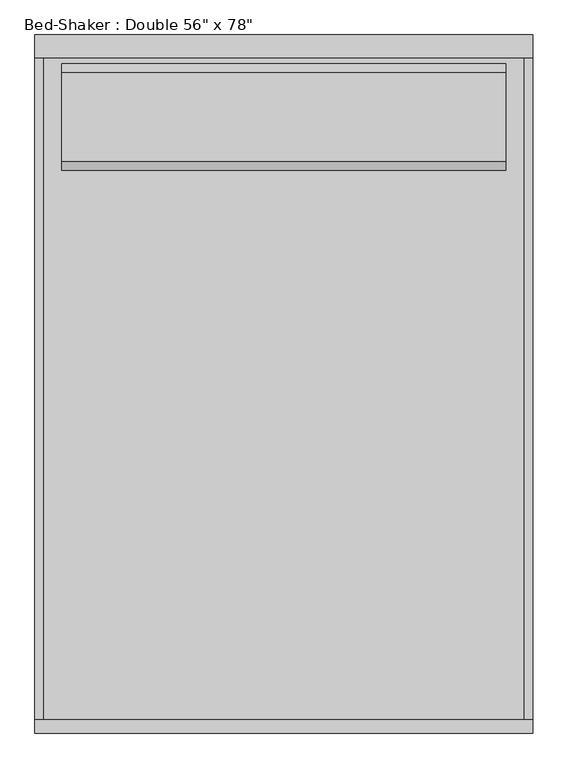
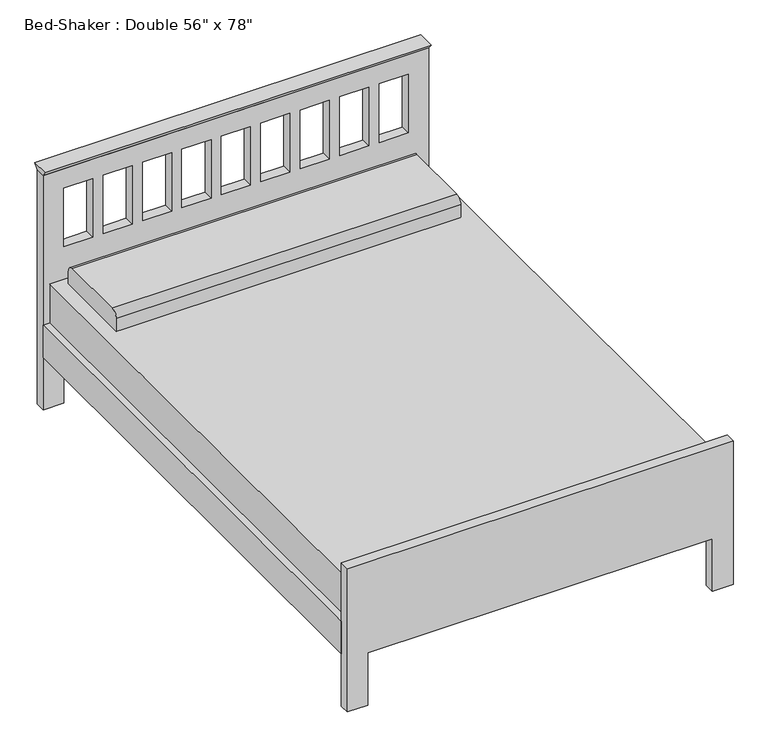
"""IFC4 building model written with IfcOpenShell, lengths in millimetres: furniture geometry."""

from ifc_helpers import new_model, si_unit, point, frame, frame_2d, origin, place, context, project, spatial, polyline, circle_curve, trimmed, segment, composite_curve, outline, extrude, source, transform, mapped, element, save


def furniture_096e7f55(model_context):
    return source(origin(), model_context, "Body", "SweptSolid", [
        extrude(outline(polyline([(-38.1, 914.4), (-51.9545455, 933.45), (13.8545455, 933.45), (0.0, 914.4), (-38.1, 914.4)])), frame((-730.0365546, 0.0, 0.0), z_axis=(1.0, 0.0, 0.0), x_axis=(0.0, 1.0, 0.0)), (0.0, 0.0, 1.0), 1422.4533613),
        extrude(outline(composite_curve([segment(polyline([(-373.2486637, 482.6), (-373.2486637, 533.4)]), True, "CONTINUOUS"), segment(trimmed(circle_curve(frame_2d((-347.8486637, 533.4)), 25.4), [point((-373.2486637, 533.4))], [point((-347.8486637, 558.8))], False, "CARTESIAN"), True, "CONTINUOUS"), segment(polyline([(-347.8486637, 558.8), (-93.8486637, 558.8)]), True, "CONTINUOUS"), segment(trimmed(circle_curve(frame_2d((-93.8486637, 533.4)), 25.4), [point((-93.8486637, 558.8))], [point((-68.4486637, 533.4))], False, "CARTESIAN"), True, "CONTINUOUS"), segment(polyline([(-68.4486637, 533.4), (-68.4486637, 482.6), (-373.2486637, 482.6)]), True, "CONTINUOUS")], self_intersect=False)), frame((-654.05, 0.0, 0.0), z_axis=(1.0, 0.0, 0.0), x_axis=(0.0, 1.0, 0.0)), (0.0, 0.0, 1.0), 1270.0),
        extrude(outline(polyline([(666.75, -38.1), (666.75, -1943.1), (-704.85, -1943.1), (-704.85, -38.1), (666.75, -38.1)])), frame((0.0, 0.0, 228.6), z_axis=(0.0, 0.0, 1.0), x_axis=(1.0, 0.0, 0.0)), (0.0, 0.0, 1.0), 254.0),
        extrude(outline(polyline([(666.75, -1943.1), (666.75, -38.1), (692.15, -38.1), (692.15, -1943.1), (666.75, -1943.1)])), frame((0.0, 0.0, 203.0994861), z_axis=(0.0, 0.0, 1.0), x_axis=(1.0, 0.0, 0.0)), (0.0, 0.0, 1.0), 127.0),
        extrude(outline(polyline([(-730.25, -1943.1), (-730.25, -38.1), (-704.85, -38.1), (-704.85, -1943.1), (-730.25, -1943.1)])), frame((0.0, 0.0, 203.5755296), z_axis=(0.0, 0.0, 1.0), x_axis=(1.0, 0.0, 0.0)), (0.0, 0.0, 1.0), 127.0),
        extrude(outline(polyline([(0.0, -654.05), (203.2, -654.05), (203.2, 615.95), (0.0, 615.95), (0.0, 692.15), (558.8, 692.15), (558.8, -730.25), (0.0, -730.25), (0.0, -654.05)])), frame((0.0, -1981.2, 0.0), z_axis=(0.0, 1.0, 0.0), x_axis=(0.0, 0.0, 1.0)), (0.0, 0.0, 1.0), 38.1),
        extrude(outline(polyline([(914.4, 692.4168067), (914.4, -730.0365546), (0.0, -730.0365546), (0.0, -654.05), (203.2, -654.05), (203.2, 615.95), (0.0, 615.95), (0.0, 692.4168067), (914.4, 692.4168067)]), holes=[polyline([(838.2, -546.8055556), (609.6, -546.8055556), (609.6, -654.05), (838.2, -654.05), (838.2, -546.8055556)]), polyline([(838.2, -401.4611111), (609.6, -401.4611111), (609.6, -508.7055556), (838.2, -508.7055556), (838.2, -401.4611111)]), polyline([(838.2, -256.1166667), (609.6, -256.1166667), (609.6, -363.3611111), (838.2, -363.3611111), (838.2, -256.1166667)]), polyline([(838.2, -110.7722222), (609.6, -110.7722222), (609.6, -218.0166667), (838.2, -218.0166667), (838.2, -110.7722222)]), polyline([(838.2, 179.9166667), (609.6, 179.9166667), (609.6, 72.6722222), (838.2, 72.6722222), (838.2, 179.9166667)]), polyline([(838.2, 325.2611111), (609.6, 325.2611111), (609.6, 218.0166667), (838.2, 218.0166667), (838.2, 325.2611111)]), polyline([(838.2, 470.6055556), (609.6, 470.6055556), (609.6, 363.3611111), (838.2, 363.3611111), (838.2, 470.6055556)]), polyline([(838.2, 615.95), (609.6, 615.95), (609.6, 508.7055556), (838.2, 508.7055556), (838.2, 615.95)]), polyline([(838.2, 34.5722222), (609.6, 34.5722222), (609.6, -72.6722222), (838.2, -72.6722222), (838.2, 34.5722222)])]), frame((0.0, -38.1, 0.0), z_axis=(0.0, 1.0, 0.0), x_axis=(0.0, 0.0, 1.0)), (0.0, 0.0, 1.0), 38.1),
    ])


if __name__ == "__main__":
    model = new_model("IFC4")
    model_context = context("Model", 3, world=origin())
    ifc_project = project(units=[si_unit("LENGTHUNIT", "METRE", prefix="MILLI")], contexts=[model_context])
    site = spatial("IfcSite", under=ifc_project)
    building = spatial("IfcBuilding", under=site)
    placement = place(None, origin())
    furniture_shape = furniture_096e7f55(model_context)
    element("IfcFurniture", 1, ObjectType="Bed-Shaker : Double 56\" x 78\"", at=placement, inside=building, context=model_context, shape_type="MappedRepresentation", body=[
        mapped(furniture_shape, transform((0.0, 0.0, 0.0), x_axis=(1.0, 0.0, 0.0), y_axis=(0.0, 1.0, 0.0), z_axis=(0.0, 0.0, 1.0))),
    ])
    save(model, "model.ifc")

# Revit data of these elements
# Type "Bed-Shaker : Double 56\" x 78\""
#   Assembly Code = "E2020200"
#   Length = 6' - 6"
#   Width = 4' - 8"
#   Frame Material = Birch
#   Mattress Material = Plywood, Sheathing
#   Default Elevation = 0
# Element 1 (IfcFurniture, "Bed-Shaker : Double 56\" x 78\"")
#   Materials on its faces: "Birch", "Plywood, Sheathing"
# Materials
#   "Birch": class "Wood", colour RGB 224 178 126, transparency 0, Description = "Betula Alleghaniensis", Cost = 0
#   "Plywood, Sheathing": class "Wood", colour RGB 212 179 113, transparency 0, Description = "Plywood, sheathing grade", Cost = 0
